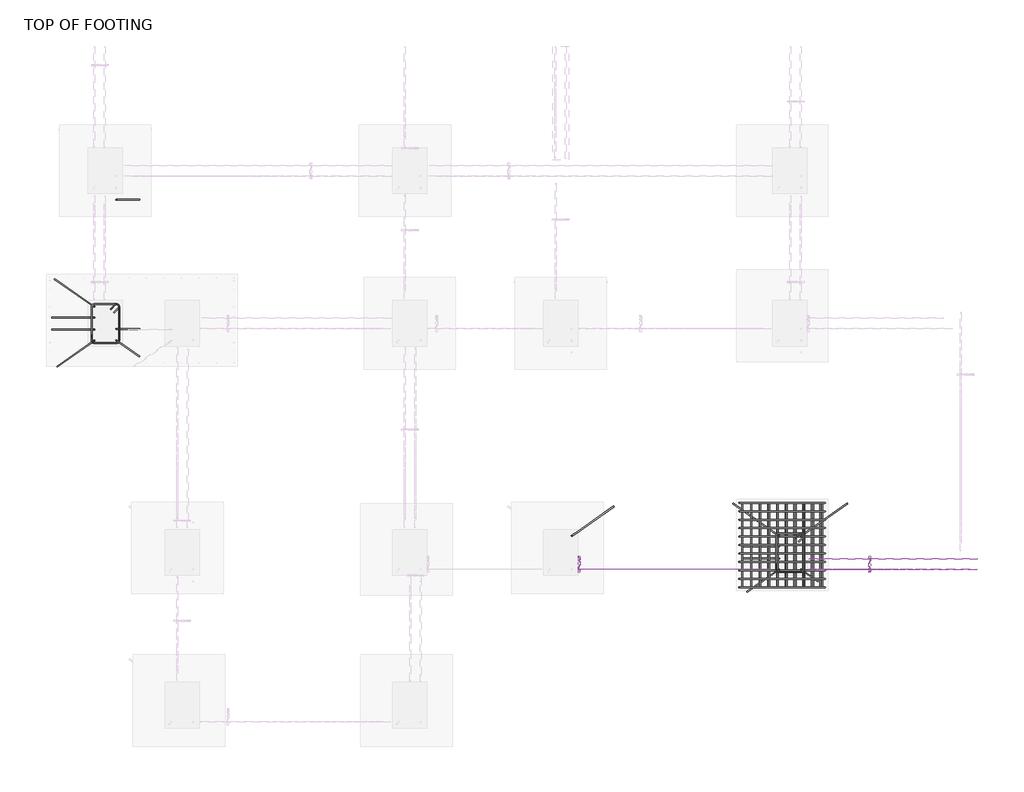
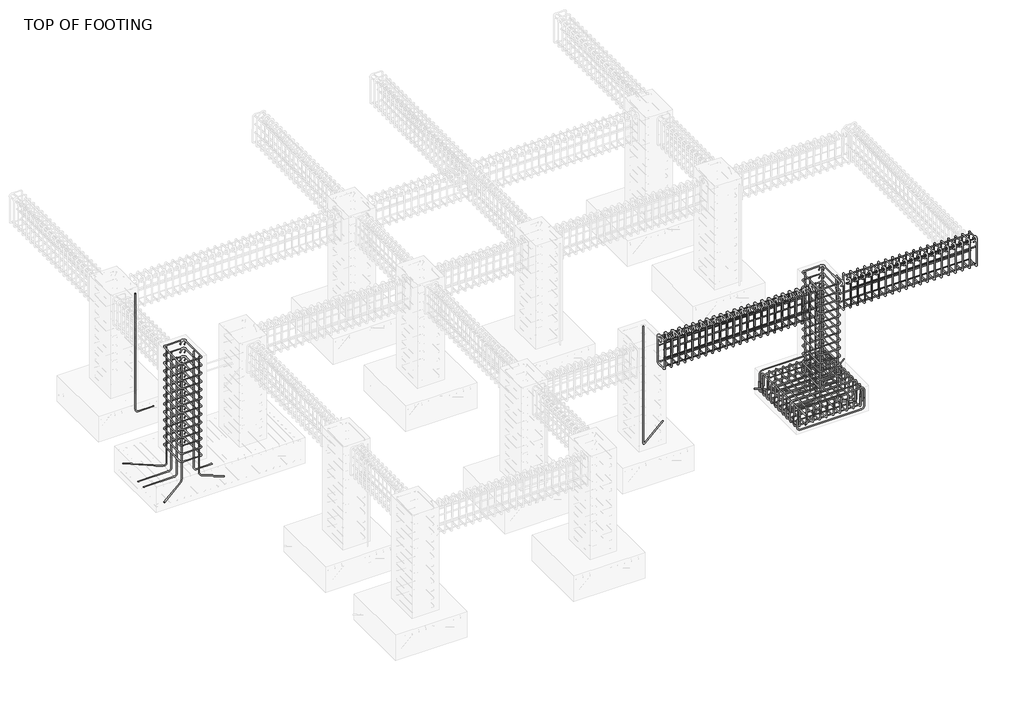
# One storey, part 5 of 17: 27 reinforcing bars.
"""IFC4 building model written with IfcOpenShell, lengths in millimetres."""

from ifc_helpers import new_model, si_unit, point, frame, origin, place, context, project, spatial, polyline, circle_curve, trimmed, segment, composite_curve, source, transform, mapped, element, save
from ifc_brep_helpers import swept_disk

model = new_model("IFC4")

# Units and contexts
model_context = context("Model", 3, world=origin())
ifc_project = project(units=[si_unit("LENGTHUNIT", "METRE", prefix="MILLI")], contexts=[model_context])

# Site, building, storey
site = spatial("IfcSite", under=ifc_project)
building = spatial("IfcBuilding", under=site)
storey = spatial("IfcBuildingStorey", under=building, Name="TOP OF FOOTING", Elevation=-1828.8)

# Reinforcing bars
placement = place(None, origin())
reinforcing_bar_shape = source(origin(), model_context, "Body", "SolidModel", [
    swept_disk(composite_curve([segment(polyline([(5115.7588658, -280.8742842, -2051.4362487), (5115.7588658, -280.8742842, -2198.7362487)]), True, "CONTINUOUS"), segment(trimmed(circle_curve(frame((5069.4088658, -280.8742842, -2198.7362487), z_axis=(0.0, 1.0, 0.0), x_axis=(46.350000000000364, 0.0, 0.0)), 46.35), [point((5115.7588658, -280.8742842, -2198.7362487))], [point((5069.4088658, -280.8742842, -2245.0862487))], True, "CARTESIAN"), True, "CONTINUOUS"), segment(polyline([(5069.4088658, -280.8742842, -2245.0862487), (4044.0910413, -280.8742842, -2245.0862487)]), True, "CONTINUOUS"), segment(trimmed(circle_curve(frame((4044.0910413, -280.8742842, -2198.7362487), z_axis=(0.0, 1.0, 0.0), x_axis=(0.0, 0.0, -46.34999999999991)), 46.35), [point((4044.0910413, -280.8742842, -2245.0862487))], [point((3997.7410413, -280.8742842, -2198.7362487))], True, "CARTESIAN"), True, "CONTINUOUS"), segment(polyline([(3997.7410413, -280.8742842, -2198.7362487), (3997.7410413, -280.8742842, -2051.4362487)]), True, "CONTINUOUS")], self_intersect=False), 6.35),
])
element("IfcReinforcingBar", 1, at=placement, inside=storey, context=model_context, shape_type="MappedRepresentation", body=[
    mapped(reinforcing_bar_shape, transform((0.0, 0.0, 0.0), x_axis=(1.0, 0.0, 0.0), y_axis=(0.0, 1.0, 0.0), z_axis=(0.0, 0.0, 1.0))),
    mapped(reinforcing_bar_shape, transform((0.0, -110.73, 0.0), x_axis=(1.0, 0.0, 0.0), y_axis=(0.0, 1.0, 0.0), z_axis=(0.0, 0.0, 1.0))),
    mapped(reinforcing_bar_shape, transform((0.0, -221.46, 0.0), x_axis=(1.0, 0.0, 0.0), y_axis=(0.0, 1.0, 0.0), z_axis=(0.0, 0.0, 1.0))),
    mapped(reinforcing_bar_shape, transform((0.0, -332.19, 0.0), x_axis=(1.0, 0.0, 0.0), y_axis=(0.0, 1.0, 0.0), z_axis=(0.0, 0.0, 1.0))),
    mapped(reinforcing_bar_shape, transform((0.0, -442.92, 0.0), x_axis=(1.0, 0.0, 0.0), y_axis=(0.0, 1.0, 0.0), z_axis=(0.0, 0.0, 1.0))),
    mapped(reinforcing_bar_shape, transform((0.0, -553.65, 0.0), x_axis=(1.0, 0.0, 0.0), y_axis=(0.0, 1.0, 0.0), z_axis=(0.0, 0.0, 1.0))),
    mapped(reinforcing_bar_shape, transform((0.0, -664.38, 0.0), x_axis=(1.0, 0.0, 0.0), y_axis=(0.0, 1.0, 0.0), z_axis=(0.0, 0.0, 1.0))),
    mapped(reinforcing_bar_shape, transform((0.0, -775.11, 0.0), x_axis=(1.0, 0.0, 0.0), y_axis=(0.0, 1.0, 0.0), z_axis=(0.0, 0.0, 1.0))),
    mapped(reinforcing_bar_shape, transform((0.0, -885.84, 0.0), x_axis=(1.0, 0.0, 0.0), y_axis=(0.0, 1.0, 0.0), z_axis=(0.0, 0.0, 1.0))),
    mapped(reinforcing_bar_shape, transform((0.0, -996.57, 0.0), x_axis=(1.0, 0.0, 0.0), y_axis=(0.0, 1.0, 0.0), z_axis=(0.0, 0.0, 1.0))),
    mapped(reinforcing_bar_shape, transform((0.0, -1107.3, 0.0), x_axis=(1.0, 0.0, 0.0), y_axis=(0.0, 1.0, 0.0), z_axis=(0.0, 0.0, 1.0))),
])
reinforcing_bar_2_shape = source(origin(), model_context, "Body", "SolidModel", [
    swept_disk(composite_curve([segment(polyline([(4008.404705, -280.8742842, -2058.517229), (4008.404705, -280.8742842, -1911.217229)]), True, "CONTINUOUS"), segment(trimmed(circle_curve(frame((4054.754705, -280.8742842, -1911.217229), z_axis=(0.0, 1.0, 0.0), x_axis=(-46.34999999999991, 0.0, 0.0)), 46.35), [point((4008.404705, -280.8742842, -1911.217229))], [point((4054.754705, -280.8742842, -1864.867229))], True, "CARTESIAN"), True, "CONTINUOUS"), segment(polyline([(4054.754705, -280.8742842, -1864.867229), (5073.3110915, -280.8742842, -1864.867229)]), True, "CONTINUOUS"), segment(trimmed(circle_curve(frame((5073.3110915, -280.8742842, -1911.217229), z_axis=(0.0, 1.0, 0.0), x_axis=(0.0, 0.0, 46.350000000000136)), 46.35), [point((5073.3110915, -280.8742842, -1864.867229))], [point((5119.6610915, -280.8742842, -1911.217229))], True, "CARTESIAN"), True, "CONTINUOUS"), segment(polyline([(5119.6610915, -280.8742842, -1911.217229), (5119.6610915, -280.8742842, -2058.517229)]), True, "CONTINUOUS")], self_intersect=False), 6.35),
])
element("IfcReinforcingBar", 2, at=placement, inside=storey, context=model_context, shape_type="MappedRepresentation", body=[
    mapped(reinforcing_bar_2_shape, transform((0.0, 0.0, 0.0), x_axis=(1.0, 0.0, 0.0), y_axis=(0.0, 1.0, 0.0), z_axis=(0.0, 0.0, 1.0))),
    mapped(reinforcing_bar_2_shape, transform((0.0, -110.73, 0.0), x_axis=(1.0, 0.0, 0.0), y_axis=(0.0, 1.0, 0.0), z_axis=(0.0, 0.0, 1.0))),
    mapped(reinforcing_bar_2_shape, transform((0.0, -221.46, 0.0), x_axis=(1.0, 0.0, 0.0), y_axis=(0.0, 1.0, 0.0), z_axis=(0.0, 0.0, 1.0))),
    mapped(reinforcing_bar_2_shape, transform((0.0, -332.19, 0.0), x_axis=(1.0, 0.0, 0.0), y_axis=(0.0, 1.0, 0.0), z_axis=(0.0, 0.0, 1.0))),
    mapped(reinforcing_bar_2_shape, transform((0.0, -442.92, 0.0), x_axis=(1.0, 0.0, 0.0), y_axis=(0.0, 1.0, 0.0), z_axis=(0.0, 0.0, 1.0))),
    mapped(reinforcing_bar_2_shape, transform((0.0, -553.65, 0.0), x_axis=(1.0, 0.0, 0.0), y_axis=(0.0, 1.0, 0.0), z_axis=(0.0, 0.0, 1.0))),
    mapped(reinforcing_bar_2_shape, transform((0.0, -664.38, 0.0), x_axis=(1.0, 0.0, 0.0), y_axis=(0.0, 1.0, 0.0), z_axis=(0.0, 0.0, 1.0))),
    mapped(reinforcing_bar_2_shape, transform((0.0, -775.11, 0.0), x_axis=(1.0, 0.0, 0.0), y_axis=(0.0, 1.0, 0.0), z_axis=(0.0, 0.0, 1.0))),
    mapped(reinforcing_bar_2_shape, transform((0.0, -885.84, 0.0), x_axis=(1.0, 0.0, 0.0), y_axis=(0.0, 1.0, 0.0), z_axis=(0.0, 0.0, 1.0))),
    mapped(reinforcing_bar_2_shape, transform((0.0, -996.57, 0.0), x_axis=(1.0, 0.0, 0.0), y_axis=(0.0, 1.0, 0.0), z_axis=(0.0, 0.0, 1.0))),
    mapped(reinforcing_bar_2_shape, transform((0.0, -1107.3, 0.0), x_axis=(1.0, 0.0, 0.0), y_axis=(0.0, 1.0, 0.0), z_axis=(0.0, 0.0, 1.0))),
])
reinforcing_bar_3_shape = source(origin(), model_context, "Body", "SolidModel", [
    swept_disk(composite_curve([segment(polyline([(5082.6693864, -280.8742842, -2093.0974099), (5082.6693864, -280.8742842, -1945.7974099)]), True, "CONTINUOUS"), segment(trimmed(circle_curve(frame((5082.6693864, -327.2242842, -1945.7974099), z_axis=(1.0, 0.0, 0.0), x_axis=(0.0, 46.35000000000002, 0.0)), 46.35), [point((5082.6693864, -280.8742842, -1945.7974099))], [point((5082.6693864, -327.2242842, -1899.4474099))], True, "CARTESIAN"), True, "CONTINUOUS"), segment(polyline([(5082.6693864, -327.2242842, -1899.4474099), (5082.6693864, -1341.8242842, -1899.4474099)]), True, "CONTINUOUS"), segment(trimmed(circle_curve(frame((5082.6693864, -1341.8242842, -1945.7974099), z_axis=(1.0, 0.0, 0.0), x_axis=(0.0, 0.0, 46.350000000000136)), 46.35), [point((5082.6693864, -1341.8242842, -1899.4474099))], [point((5082.6693864, -1388.1742842, -1945.7974099))], True, "CARTESIAN"), True, "CONTINUOUS"), segment(polyline([(5082.6693864, -1388.1742842, -1945.7974099), (5082.6693864, -1388.1742842, -2093.0974099)]), True, "CONTINUOUS")], self_intersect=False), 6.35),
])
element("IfcReinforcingBar", 3, at=placement, inside=storey, context=model_context, shape_type="MappedRepresentation", body=[
    mapped(reinforcing_bar_3_shape, transform((0.0, 0.0, 0.0), x_axis=(1.0, 0.0, 0.0), y_axis=(0.0, 1.0, 0.0), z_axis=(0.0, 0.0, 1.0))),
    mapped(reinforcing_bar_3_shape, transform((-115.9606781, 0.0, 0.0), x_axis=(1.0, 0.0, 0.0), y_axis=(0.0, 1.0, 0.0), z_axis=(0.0, 0.0, 1.0))),
    mapped(reinforcing_bar_3_shape, transform((-231.9213561, 0.0, 0.0), x_axis=(1.0, 0.0, 0.0), y_axis=(0.0, 1.0, 0.0), z_axis=(0.0, 0.0, 1.0))),
    mapped(reinforcing_bar_3_shape, transform((-347.8820342, 0.0, 0.0), x_axis=(1.0, 0.0, 0.0), y_axis=(0.0, 1.0, 0.0), z_axis=(0.0, 0.0, 1.0))),
    mapped(reinforcing_bar_3_shape, transform((-463.8427123, 0.0, 0.0), x_axis=(1.0, 0.0, 0.0), y_axis=(0.0, 1.0, 0.0), z_axis=(0.0, 0.0, 1.0))),
    mapped(reinforcing_bar_3_shape, transform((-579.8033904, 0.0, 0.0), x_axis=(1.0, 0.0, 0.0), y_axis=(0.0, 1.0, 0.0), z_axis=(0.0, 0.0, 1.0))),
    mapped(reinforcing_bar_3_shape, transform((-695.7640684, 0.0, 0.0), x_axis=(1.0, 0.0, 0.0), y_axis=(0.0, 1.0, 0.0), z_axis=(0.0, 0.0, 1.0))),
    mapped(reinforcing_bar_3_shape, transform((-811.7247465, 0.0, 0.0), x_axis=(1.0, 0.0, 0.0), y_axis=(0.0, 1.0, 0.0), z_axis=(0.0, 0.0, 1.0))),
    mapped(reinforcing_bar_3_shape, transform((-927.6854246, 0.0, 0.0), x_axis=(1.0, 0.0, 0.0), y_axis=(0.0, 1.0, 0.0), z_axis=(0.0, 0.0, 1.0))),
    mapped(reinforcing_bar_3_shape, transform((-1043.6461027, 0.0, 0.0), x_axis=(1.0, 0.0, 0.0), y_axis=(0.0, 1.0, 0.0), z_axis=(0.0, 0.0, 1.0))),
])
reinforcing_bar_4_shape = source(origin(), model_context, "Body", "SolidModel", [
    swept_disk(composite_curve([segment(polyline([(4039.0232837, -280.8742842, -2009.4698822), (4039.0232837, -280.8742842, -2156.7698822)]), True, "CONTINUOUS"), segment(trimmed(circle_curve(frame((4039.0232837, -327.2242842, -2156.7698822), z_axis=(-1.0, 0.0, 0.0), x_axis=(0.0, 46.35000000000002, 0.0)), 46.35), [point((4039.0232837, -280.8742842, -2156.7698822))], [point((4039.0232837, -327.2242842, -2203.1198822))], True, "CARTESIAN"), True, "CONTINUOUS"), segment(polyline([(4039.0232837, -327.2242842, -2203.1198822), (4039.0232837, -1341.8242842, -2203.1198822)]), True, "CONTINUOUS"), segment(trimmed(circle_curve(frame((4039.0232837, -1341.8242842, -2156.7698822), z_axis=(-1.0, 0.0, 0.0), x_axis=(0.0, 0.0, -46.34999999999991)), 46.35), [point((4039.0232837, -1341.8242842, -2203.1198822))], [point((4039.0232837, -1388.1742842, -2156.7698822))], True, "CARTESIAN"), True, "CONTINUOUS"), segment(polyline([(4039.0232837, -1388.1742842, -2156.7698822), (4039.0232837, -1388.1742842, -2009.4698822)]), True, "CONTINUOUS")], self_intersect=False), 6.35),
])
element("IfcReinforcingBar", 4, at=placement, inside=storey, context=model_context, shape_type="MappedRepresentation", body=[
    mapped(reinforcing_bar_4_shape, transform((0.0, 0.0, 0.0), x_axis=(1.0, 0.0, 0.0), y_axis=(0.0, 1.0, 0.0), z_axis=(0.0, 0.0, 1.0))),
    mapped(reinforcing_bar_4_shape, transform((113.1523491, 0.0, 0.0), x_axis=(1.0, 0.0, 0.0), y_axis=(0.0, 1.0, 0.0), z_axis=(0.0, 0.0, 1.0))),
    mapped(reinforcing_bar_4_shape, transform((226.3046983, 0.0, 0.0), x_axis=(1.0, 0.0, 0.0), y_axis=(0.0, 1.0, 0.0), z_axis=(0.0, 0.0, 1.0))),
    mapped(reinforcing_bar_4_shape, transform((339.4570474, 0.0, 0.0), x_axis=(1.0, 0.0, 0.0), y_axis=(0.0, 1.0, 0.0), z_axis=(0.0, 0.0, 1.0))),
    mapped(reinforcing_bar_4_shape, transform((452.6093966, 0.0, 0.0), x_axis=(1.0, 0.0, 0.0), y_axis=(0.0, 1.0, 0.0), z_axis=(0.0, 0.0, 1.0))),
    mapped(reinforcing_bar_4_shape, transform((565.7617457, 0.0, 0.0), x_axis=(1.0, 0.0, 0.0), y_axis=(0.0, 1.0, 0.0), z_axis=(0.0, 0.0, 1.0))),
    mapped(reinforcing_bar_4_shape, transform((678.9140949, 0.0, 0.0), x_axis=(1.0, 0.0, 0.0), y_axis=(0.0, 1.0, 0.0), z_axis=(0.0, 0.0, 1.0))),
    mapped(reinforcing_bar_4_shape, transform((792.066444, 0.0, 0.0), x_axis=(1.0, 0.0, 0.0), y_axis=(0.0, 1.0, 0.0), z_axis=(0.0, 0.0, 1.0))),
    mapped(reinforcing_bar_4_shape, transform((905.2187932, 0.0, 0.0), x_axis=(1.0, 0.0, 0.0), y_axis=(0.0, 1.0, 0.0), z_axis=(0.0, 0.0, 1.0))),
    mapped(reinforcing_bar_4_shape, transform((1018.3711423, 0.0, 0.0), x_axis=(1.0, 0.0, 0.0), y_axis=(0.0, 1.0, 0.0), z_axis=(0.0, 0.0, 1.0))),
])
reinforcing_bar_5_shape = source(origin(), model_context, "Body", "SolidModel", [
    swept_disk(composite_curve([segment(polyline([(-4230.403382, 2254.1999505, -46.35), (-4174.6598191, 2309.9435134, -46.35)]), True, "CONTINUOUS"), segment(trimmed(circle_curve(frame((-4152.4920215, 2287.7757158, -46.35), z_axis=(0.0, 0.0, -1.0), x_axis=(-22.167797600000085, 22.167797600000085, 0.0)), 31.35), [point((-4174.6598191, 2309.9435134, -46.35))], [point((-4121.1420215, 2287.7757158, -46.35))], True, "CARTESIAN"), True, "CONTINUOUS"), segment(polyline([(-4121.1420215, 2287.7757158, -46.35), (-4121.1420215, 1843.1757158, -46.35)]), True, "CONTINUOUS"), segment(trimmed(circle_curve(frame((-4152.4920215, 1843.1757158, -46.35), z_axis=(0.0, 0.0, -1.0), x_axis=(31.350000000000364, 0.0, 0.0)), 31.35), [point((-4121.1420215, 1843.1757158, -46.35))], [point((-4152.4920215, 1811.8257158, -46.35))], True, "CARTESIAN"), True, "CONTINUOUS"), segment(polyline([(-4152.4920215, 1811.8257158, -46.35), (-4447.0920215, 1811.8257158, -46.35)]), True, "CONTINUOUS"), segment(trimmed(circle_curve(frame((-4447.0920215, 1843.1658965, -45.5654144), z_axis=(0.0, 0.025026655153786343, -0.9996867842138424), x_axis=(0.0, -31.34018070000002, -0.7845855999999998)), 31.35), [point((-4447.0920215, 1811.8257158, -46.35))], [point((-4478.4420215, 1843.1658965, -45.5654144))], True, "CARTESIAN"), True, "CONTINUOUS"), segment(polyline([(-4478.4420215, 1843.1658965, -45.5654144), (-4478.4420215, 2287.7855351, -34.4345856)]), True, "CONTINUOUS"), segment(trimmed(circle_curve(frame((-4447.0920215, 2287.7855351, -34.4345856), z_axis=(0.0, 0.025026655153786343, -0.9996867842138424), x_axis=(-31.350000000000364, 0.0, 0.0)), 31.35), [point((-4478.4420215, 2287.7855351, -34.4345856))], [point((-4447.0920215, 2319.1257158, -33.65))], True, "CARTESIAN"), True, "CONTINUOUS"), segment(polyline([(-4447.0920215, 2319.1257158, -33.65), (-4152.4920215, 2319.1257158, -33.65)]), True, "CONTINUOUS"), segment(trimmed(circle_curve(frame((-4152.4920215, 2287.7757158, -33.65), z_axis=(0.0, 0.0, -1.0), x_axis=(0.0, 31.34999999999991, 0.0)), 31.35), [point((-4152.4920215, 2319.1257158, -33.65))], [point((-4130.3242239, 2265.6079182, -33.65))], True, "CARTESIAN"), True, "CONTINUOUS"), segment(polyline([(-4130.3242239, 2265.6079182, -33.65), (-4186.0677868, 2209.8643553, -33.65)]), True, "CONTINUOUS")], self_intersect=False), 6.35),
])
element("IfcReinforcingBar", 5, at=placement, inside=storey, context=model_context, shape_type="MappedRepresentation", body=[
    mapped(reinforcing_bar_5_shape, transform((0.0, 0.0, 0.0), x_axis=(1.0, 0.0, 0.0), y_axis=(0.0, 1.0, 0.0), z_axis=(0.0, 0.0, 1.0))),
    mapped(reinforcing_bar_5_shape, transform((0.0, 0.0, -144.675), x_axis=(1.0, 0.0, 0.0), y_axis=(0.0, 1.0, 0.0), z_axis=(0.0, 0.0, 1.0))),
    mapped(reinforcing_bar_5_shape, transform((0.0, 0.0, -289.35), x_axis=(1.0, 0.0, 0.0), y_axis=(0.0, 1.0, 0.0), z_axis=(0.0, 0.0, 1.0))),
    mapped(reinforcing_bar_5_shape, transform((0.0, 0.0, -434.025), x_axis=(1.0, 0.0, 0.0), y_axis=(0.0, 1.0, 0.0), z_axis=(0.0, 0.0, 1.0))),
    mapped(reinforcing_bar_5_shape, transform((0.0, 0.0, -578.7), x_axis=(1.0, 0.0, 0.0), y_axis=(0.0, 1.0, 0.0), z_axis=(0.0, 0.0, 1.0))),
    mapped(reinforcing_bar_5_shape, transform((0.0, 0.0, -723.375), x_axis=(1.0, 0.0, 0.0), y_axis=(0.0, 1.0, 0.0), z_axis=(0.0, 0.0, 1.0))),
    mapped(reinforcing_bar_5_shape, transform((0.0, 0.0, -868.05), x_axis=(1.0, 0.0, 0.0), y_axis=(0.0, 1.0, 0.0), z_axis=(0.0, 0.0, 1.0))),
    mapped(reinforcing_bar_5_shape, transform((0.0, 0.0, -1012.725), x_axis=(1.0, 0.0, 0.0), y_axis=(0.0, 1.0, 0.0), z_axis=(0.0, 0.0, 1.0))),
    mapped(reinforcing_bar_5_shape, transform((0.0, 0.0, -1157.4), x_axis=(1.0, 0.0, 0.0), y_axis=(0.0, 1.0, 0.0), z_axis=(0.0, 0.0, 1.0))),
    mapped(reinforcing_bar_5_shape, transform((0.0, 0.0, -1302.075), x_axis=(1.0, 0.0, 0.0), y_axis=(0.0, 1.0, 0.0), z_axis=(0.0, 0.0, 1.0))),
    mapped(reinforcing_bar_5_shape, transform((0.0, 0.0, -1446.75), x_axis=(1.0, 0.0, 0.0), y_axis=(0.0, 1.0, 0.0), z_axis=(0.0, 0.0, 1.0))),
    mapped(reinforcing_bar_5_shape, transform((0.0, 0.0, -1591.425), x_axis=(1.0, 0.0, 0.0), y_axis=(0.0, 1.0, 0.0), z_axis=(0.0, 0.0, 1.0))),
    mapped(reinforcing_bar_5_shape, transform((0.0, 0.0, -1736.1), x_axis=(1.0, 0.0, 0.0), y_axis=(0.0, 1.0, 0.0), z_axis=(0.0, 0.0, 1.0))),
])
reinforcing_bar_6_shape = source(origin(), model_context, "Body", "SolidModel", [
    swept_disk(composite_curve([segment(polyline([(-4155.5276111, 1997.3689995, -40.0), (-4155.5276111, 1997.3689995, -2094.5391135)]), True, "CONTINUOUS"), segment(trimmed(circle_curve(frame((-4109.1776111, 1997.3689995, -2094.5391135), z_axis=(0.0, -1.0, 0.0), x_axis=(-46.350000000000364, 0.0, 0.0)), 46.35), [point((-4155.5276111, 1997.3689995, -2094.5391135))], [point((-4109.1776111, 1997.3689995, -2140.8891135))], True, "CARTESIAN"), True, "CONTINUOUS"), segment(polyline([(-4109.1776111, 1997.3689995, -2140.8891135), (-3849.2038294, 1997.3689995, -2140.8891135)]), True, "CONTINUOUS")], self_intersect=False), 6.35),
])
element("IfcReinforcingBar", 6, at=placement, inside=storey, context=model_context, shape_type="MappedRepresentation", body=[
    mapped(reinforcing_bar_6_shape, transform((0.0, 0.0, 0.0), x_axis=(1.0, 0.0, 0.0), y_axis=(0.0, 1.0, 0.0), z_axis=(0.0, 0.0, 1.0))),
    mapped(reinforcing_bar_6_shape, transform((0.0, 1690.7260472, 0.0), x_axis=(1.0, 0.0, 0.0), y_axis=(0.0, 1.0, 0.0), z_axis=(0.0, 0.0, 1.0))),
])
element("IfcReinforcingBar", 7, at=placement, inside=storey, context=model_context, shape_type="SolidModel", body=[
    swept_disk(composite_curve([segment(polyline([(-4444.0564318, 2286.4257158, -40.0), (-4444.0564318, 2286.4257158, -2094.5391135)]), True, "CONTINUOUS"), segment(trimmed(circle_curve(frame((-4482.0241291, 2313.0109836, -2094.5391135), z_axis=(0.5735764363510419, 0.8191520442889948, 0.0), x_axis=(37.96769730000051, -26.58526780000011, 0.0)), 46.35), [point((-4444.0564318, 2286.4257158, -2094.5391135))], [point((-4482.0241291, 2313.0109836, -2140.8891135))], True, "CARTESIAN"), True, "CONTINUOUS"), segment(polyline([(-4482.0241291, 2313.0109836, -2140.8891135), (-4963.5335446, 2650.1675061, -2140.8891135)]), True, "CONTINUOUS")], self_intersect=False), 6.35),
])
element("IfcReinforcingBar", 8, at=placement, inside=storey, context=model_context, shape_type="SolidModel", body=[
    swept_disk(composite_curve([segment(polyline([(-4155.5276111, 1844.5257158, -40.0), (-4155.5276111, 1844.5257158, -2094.5391135)]), True, "CONTINUOUS"), segment(trimmed(circle_curve(frame((-4117.5599139, 1817.940448, -2094.5391135), z_axis=(-0.5735764363510363, -0.8191520442889988, 0.0), x_axis=(-37.96769720000066, 26.585267799999883, 0.0)), 46.35), [point((-4155.5276111, 1844.5257158, -2094.5391135))], [point((-4117.5599139, 1817.940448, -2140.8891135))], True, "CARTESIAN"), True, "CONTINUOUS"), segment(polyline([(-4117.5599139, 1817.940448, -2140.8891135), (-3853.7755504, 1633.2366482, -2140.8891135)]), True, "CONTINUOUS")], self_intersect=False), 6.35),
])
element("IfcReinforcingBar", 9, at=placement, inside=storey, context=model_context, shape_type="SolidModel", body=[
    swept_disk(composite_curve([segment(polyline([(-4444.0564318, 1844.5257158, -40.0), (-4444.0564318, 1844.5257158, -2094.5391135)]), True, "CONTINUOUS"), segment(trimmed(circle_curve(frame((-4482.0241291, 1817.940448, -2094.5391135), z_axis=(-0.5735764363510419, 0.8191520442889948, 0.0), x_axis=(37.96769730000051, 26.585267799999883, 0.0)), 46.35), [point((-4444.0564318, 1844.5257158, -2094.5391135))], [point((-4482.0241291, 1817.940448, -2140.8891135))], True, "CARTESIAN"), True, "CONTINUOUS"), segment(polyline([(-4482.0241291, 1817.940448, -2140.8891135), (-4933.5928236, 1501.748644, -2140.8891135)]), True, "CONTINUOUS")], self_intersect=False), 6.35),
])
reinforcing_bar_7_shape = source(origin(), model_context, "Body", "SolidModel", [
    swept_disk(composite_curve([segment(polyline([(-4444.0564318, 2147.3689995, -40.0), (-4444.0564318, 2147.3689995, -2094.5391135)]), True, "CONTINUOUS"), segment(trimmed(circle_curve(frame((-4490.4064318, 2147.3689995, -2094.5391135), z_axis=(0.0, 1.0, 0.0), x_axis=(46.350000000000364, 0.0, 0.0)), 46.35), [point((-4444.0564318, 2147.3689995, -2094.5391135))], [point((-4490.4064318, 2147.3689995, -2140.8891135))], True, "CARTESIAN"), True, "CONTINUOUS"), segment(polyline([(-4490.4064318, 2147.3689995, -2140.8891135), (-5004.1383392, 2147.3689995, -2140.8891135)]), True, "CONTINUOUS")], self_intersect=False), 6.35),
])
element("IfcReinforcingBar", 10, at=placement, inside=storey, context=model_context, shape_type="MappedRepresentation", body=[
    mapped(reinforcing_bar_7_shape, transform((0.0, 0.0, 0.0), x_axis=(1.0, 0.0, 0.0), y_axis=(0.0, 1.0, 0.0), z_axis=(0.0, 0.0, 1.0))),
    mapped(reinforcing_bar_7_shape, transform((0.0, -159.2739528, 0.0), x_axis=(1.0, 0.0, 0.0), y_axis=(0.0, 1.0, 0.0), z_axis=(0.0, 0.0, 1.0))),
])
element("IfcReinforcingBar", 11, at=placement, inside=storey, context=model_context, shape_type="SolidModel", body=[
    swept_disk(composite_curve([segment(polyline([(1806.3732761, -713.5742842, -40.0), (1806.3732761, -713.5742842, -2094.5391135)]), True, "CONTINUOUS"), segment(trimmed(circle_curve(frame((1844.3409734, -686.9890164, -2094.5391135), z_axis=(0.5735764363510363, -0.8191520442889988, 0.0), x_axis=(-37.96769729999983, -26.585267799999997, 0.0)), 46.35), [point((1806.3732761, -713.5742842, -2094.5391135))], [point((1844.3409734, -686.9890164, -2140.8891135))], True, "CARTESIAN"), True, "CONTINUOUS"), segment(polyline([(1844.3409734, -686.9890164, -2140.8891135), (2354.4133491, -329.8324939, -2140.8891135)]), True, "CONTINUOUS")], self_intersect=False), 6.35),
])
reinforcing_bar_8_shape = source(origin(), model_context, "Body", "SolidModel", [
    swept_disk(composite_curve([segment(polyline([(4731.4975053, -745.8000495, -46.35), (4787.2410682, -690.0564866, -46.35)]), True, "CONTINUOUS"), segment(trimmed(circle_curve(frame((4809.4088658, -712.2242842, -46.35), z_axis=(0.0, 0.0, -1.0), x_axis=(-22.167797600000085, 22.167797600000085, 0.0)), 31.35), [point((4787.2410682, -690.0564866, -46.35))], [point((4840.7588658, -712.2242842, -46.35))], True, "CARTESIAN"), True, "CONTINUOUS"), segment(polyline([(4840.7588658, -712.2242842, -46.35), (4840.7588658, -1156.8242842, -46.35)]), True, "CONTINUOUS"), segment(trimmed(circle_curve(frame((4809.4088658, -1156.8242842, -46.35), z_axis=(0.0, 0.0, -1.0), x_axis=(31.350000000000364, 0.0, 0.0)), 31.35), [point((4840.7588658, -1156.8242842, -46.35))], [point((4809.4088658, -1188.1742842, -46.35))], True, "CARTESIAN"), True, "CONTINUOUS"), segment(polyline([(4809.4088658, -1188.1742842, -46.35), (4514.8088658, -1188.1742842, -46.35)]), True, "CONTINUOUS"), segment(trimmed(circle_curve(frame((4514.8088658, -1156.8341035, -45.5654144), z_axis=(0.0, 0.025026655153786343, -0.9996867842138424), x_axis=(0.0, -31.34018070000002, -0.7845855999999998)), 31.35), [point((4514.8088658, -1188.1742842, -46.35))], [point((4483.4588658, -1156.8341035, -45.5654144))], True, "CARTESIAN"), True, "CONTINUOUS"), segment(polyline([(4483.4588658, -1156.8341035, -45.5654144), (4483.4588658, -712.2144649, -34.4345856)]), True, "CONTINUOUS"), segment(trimmed(circle_curve(frame((4514.8088658, -712.2144649, -34.4345856), z_axis=(0.0, 0.025026655153786343, -0.9996867842138424), x_axis=(-31.349999999999454, 0.0, 0.0)), 31.35), [point((4483.4588658, -712.2144649, -34.4345856))], [point((4514.8088658, -680.8742842, -33.65))], True, "CARTESIAN"), True, "CONTINUOUS"), segment(polyline([(4514.8088658, -680.8742842, -33.65), (4809.4088658, -680.8742842, -33.65)]), True, "CONTINUOUS"), segment(trimmed(circle_curve(frame((4809.4088658, -712.2242842, -33.65), z_axis=(0.0, 0.0, -1.0), x_axis=(0.0, 31.350000000000023, 0.0)), 31.35), [point((4809.4088658, -680.8742842, -33.65))], [point((4831.5766634, -734.3920818, -33.65))], True, "CARTESIAN"), True, "CONTINUOUS"), segment(polyline([(4831.5766634, -734.3920818, -33.65), (4775.8331004, -790.1356447, -33.65)]), True, "CONTINUOUS")], self_intersect=False), 6.35),
])
element("IfcReinforcingBar", 12, at=placement, inside=storey, context=model_context, shape_type="MappedRepresentation", body=[
    mapped(reinforcing_bar_8_shape, transform((0.0, 0.0, 0.0), x_axis=(1.0, 0.0, 0.0), y_axis=(0.0, 1.0, 0.0), z_axis=(0.0, 0.0, 1.0))),
    mapped(reinforcing_bar_8_shape, transform((0.0, 0.0, -144.675), x_axis=(1.0, 0.0, 0.0), y_axis=(0.0, 1.0, 0.0), z_axis=(0.0, 0.0, 1.0))),
    mapped(reinforcing_bar_8_shape, transform((0.0, 0.0, -289.35), x_axis=(1.0, 0.0, 0.0), y_axis=(0.0, 1.0, 0.0), z_axis=(0.0, 0.0, 1.0))),
    mapped(reinforcing_bar_8_shape, transform((0.0, 0.0, -434.025), x_axis=(1.0, 0.0, 0.0), y_axis=(0.0, 1.0, 0.0), z_axis=(0.0, 0.0, 1.0))),
    mapped(reinforcing_bar_8_shape, transform((0.0, 0.0, -578.7), x_axis=(1.0, 0.0, 0.0), y_axis=(0.0, 1.0, 0.0), z_axis=(0.0, 0.0, 1.0))),
    mapped(reinforcing_bar_8_shape, transform((0.0, 0.0, -723.375), x_axis=(1.0, 0.0, 0.0), y_axis=(0.0, 1.0, 0.0), z_axis=(0.0, 0.0, 1.0))),
    mapped(reinforcing_bar_8_shape, transform((0.0, 0.0, -868.05), x_axis=(1.0, 0.0, 0.0), y_axis=(0.0, 1.0, 0.0), z_axis=(0.0, 0.0, 1.0))),
    mapped(reinforcing_bar_8_shape, transform((0.0, 0.0, -1012.725), x_axis=(1.0, 0.0, 0.0), y_axis=(0.0, 1.0, 0.0), z_axis=(0.0, 0.0, 1.0))),
    mapped(reinforcing_bar_8_shape, transform((0.0, 0.0, -1157.4), x_axis=(1.0, 0.0, 0.0), y_axis=(0.0, 1.0, 0.0), z_axis=(0.0, 0.0, 1.0))),
    mapped(reinforcing_bar_8_shape, transform((0.0, 0.0, -1302.075), x_axis=(1.0, 0.0, 0.0), y_axis=(0.0, 1.0, 0.0), z_axis=(0.0, 0.0, 1.0))),
    mapped(reinforcing_bar_8_shape, transform((0.0, 0.0, -1446.75), x_axis=(1.0, 0.0, 0.0), y_axis=(0.0, 1.0, 0.0), z_axis=(0.0, 0.0, 1.0))),
    mapped(reinforcing_bar_8_shape, transform((0.0, 0.0, -1591.425), x_axis=(1.0, 0.0, 0.0), y_axis=(0.0, 1.0, 0.0), z_axis=(0.0, 0.0, 1.0))),
    mapped(reinforcing_bar_8_shape, transform((0.0, 0.0, -1736.1), x_axis=(1.0, 0.0, 0.0), y_axis=(0.0, 1.0, 0.0), z_axis=(0.0, 0.0, 1.0))),
])
element("IfcReinforcingBar", 13, at=placement, inside=storey, context=model_context, shape_type="SolidModel", body=[
    swept_disk(composite_curve([segment(polyline([(4806.3732761, -713.5742842, -40.0), (4806.3732761, -713.5742842, -2094.5391135)]), True, "CONTINUOUS"), segment(trimmed(circle_curve(frame((4844.3409734, -686.9890164, -2094.5391135), z_axis=(0.5735764363510363, -0.8191520442889988, 0.0), x_axis=(-37.9676972999996, -26.585267799999997, 0.0)), 46.35), [point((4806.3732761, -713.5742842, -2094.5391135))], [point((4844.3409734, -686.9890164, -2140.8891135))], True, "CARTESIAN"), True, "CONTINUOUS"), segment(polyline([(4844.3409734, -686.9890164, -2140.8891135), (5411.5392693, -289.8324939, -2140.8891135)]), True, "CONTINUOUS")], self_intersect=False), 6.35),
])
element("IfcReinforcingBar", 14, at=placement, inside=storey, context=model_context, shape_type="SolidModel", body=[
    swept_disk(composite_curve([segment(polyline([(4517.8444555, -713.5742842, -40.0), (4517.8444555, -713.5742842, -2094.5391135)]), True, "CONTINUOUS"), segment(trimmed(circle_curve(frame((4479.8767582, -686.9890164, -2094.5391135), z_axis=(0.5735764363510419, 0.8191520442889948, 0.0), x_axis=(37.9676972999996, -26.585267799999997, 0.0)), 46.35), [point((4517.8444555, -713.5742842, -2094.5391135))], [point((4479.8767582, -686.9890164, -2140.8891135))], True, "CARTESIAN"), True, "CONTINUOUS"), segment(polyline([(4479.8767582, -686.9890164, -2140.8891135), (3912.6784623, -289.8324939, -2140.8891135)]), True, "CONTINUOUS")], self_intersect=False), 6.35),
])
element("IfcReinforcingBar", 15, at=placement, inside=storey, context=model_context, shape_type="SolidModel", body=[
    swept_disk(composite_curve([segment(polyline([(4806.3732761, -1155.4742842, -40.0), (4806.3732761, -1155.4742842, -2094.5391135)]), True, "CONTINUOUS"), segment(trimmed(circle_curve(frame((4844.3409734, -1182.059552, -2094.5391135), z_axis=(-0.5735764363510363, -0.8191520442889988, 0.0), x_axis=(-37.9676972999996, 26.585267799999883, 0.0)), 46.35), [point((4806.3732761, -1155.4742842, -2094.5391135))], [point((4844.3409734, -1182.059552, -2140.8891135))], True, "CARTESIAN"), True, "CONTINUOUS"), segment(polyline([(4844.3409734, -1182.059552, -2140.8891135), (5025.909668, -1309.1953207, -2140.8891135)]), True, "CONTINUOUS")], self_intersect=False), 6.35),
])
element("IfcReinforcingBar", 16, at=placement, inside=storey, context=model_context, shape_type="SolidModel", body=[
    swept_disk(composite_curve([segment(polyline([(4517.8444555, -1155.4742842, -40.0), (4517.8444555, -1155.4742842, -2094.5391135)]), True, "CONTINUOUS"), segment(trimmed(circle_curve(frame((4479.8767582, -1182.059552, -2094.5391135), z_axis=(-0.5735764363510419, 0.8191520442889948, 0.0), x_axis=(37.9676972999996, 26.585267799999883, 0.0)), 46.35), [point((4517.8444555, -1155.4742842, -2094.5391135))], [point((4479.8767582, -1182.059552, -2140.8891135))], True, "CARTESIAN"), True, "CONTINUOUS"), segment(polyline([(4479.8767582, -1182.059552, -2140.8891135), (4098.3080636, -1449.2368283, -2140.8891135)]), True, "CONTINUOUS")], self_intersect=False), 6.35),
])
reinforcing_bar_9_shape = source(origin(), model_context, "Body", "SolidModel", [
    swept_disk(composite_curve([segment(polyline([(4517.8444555, -852.6310005, -40.0), (4517.8444555, -852.6310005, -2094.5391135)]), True, "CONTINUOUS"), segment(trimmed(circle_curve(frame((4471.4944555, -852.6310005, -2094.5391135), z_axis=(0.0, 1.0, 0.0), x_axis=(46.349999999999454, 0.0, 0.0)), 46.35), [point((4517.8444555, -852.6310005, -2094.5391135))], [point((4471.4944555, -852.6310005, -2140.8891135))], True, "CARTESIAN"), True, "CONTINUOUS"), segment(polyline([(4471.4944555, -852.6310005, -2140.8891135), (4027.7625481, -852.6310005, -2140.8891135)]), True, "CONTINUOUS")], self_intersect=False), 6.35),
])
element("IfcReinforcingBar", 17, at=placement, inside=storey, context=model_context, shape_type="MappedRepresentation", body=[
    mapped(reinforcing_bar_9_shape, transform((0.0, 0.0, 0.0), x_axis=(1.0, 0.0, 0.0), y_axis=(0.0, 1.0, 0.0), z_axis=(0.0, 0.0, 1.0))),
    mapped(reinforcing_bar_9_shape, transform((0.0, -159.2739528, 0.0), x_axis=(1.0, 0.0, 0.0), y_axis=(0.0, 1.0, 0.0), z_axis=(0.0, 0.0, 1.0))),
])
reinforcing_bar_10_shape = source(origin(), model_context, "Body", "SolidModel", [
    swept_disk(composite_curve([segment(polyline([(4893.4588658, -1078.9129237, -111.2757654), (4893.4588658, -1134.6564866, -55.5322024)]), True, "CONTINUOUS"), segment(trimmed(circle_curve(frame((4893.4588658, -1156.8242842, -77.7), z_axis=(1.0, 0.0, 0.0), x_axis=(0.0, 22.167797599999858, 22.1677976)), 31.35), [point((4893.4588658, -1134.6564866, -55.5322024))], [point((4893.4588658, -1188.1742842, -77.7))], True, "CARTESIAN"), True, "CONTINUOUS"), segment(polyline([(4893.4588658, -1188.1742842, -77.7), (4893.4588658, -1188.1742842, -522.3)]), True, "CONTINUOUS"), segment(trimmed(circle_curve(frame((4893.4588658, -1156.8242842, -522.3), z_axis=(1.0, 0.0, 0.0), x_axis=(0.0, -31.350000000000136, 0.0)), 31.35), [point((4893.4588658, -1188.1742842, -522.3))], [point((4893.4588658, -1156.8242842, -553.65))], True, "CARTESIAN"), True, "CONTINUOUS"), segment(polyline([(4893.4588658, -1156.8242842, -553.65), (4893.4588658, -1012.2242842, -553.65)]), True, "CONTINUOUS"), segment(trimmed(circle_curve(frame((4892.6742802, -1012.2242842, -522.3098193), z_axis=(0.9996867842138424, 0.0, 0.025026655153786322), x_axis=(0.784585600000355, 0.0, -31.34018070000002)), 31.35), [point((4893.4588658, -1012.2242842, -553.65))], [point((4892.6742802, -980.8742842, -522.3098193))], True, "CARTESIAN"), True, "CONTINUOUS"), segment(polyline([(4892.6742802, -980.8742842, -522.3098193), (4881.5434514, -980.8742842, -77.6901807)]), True, "CONTINUOUS"), segment(trimmed(circle_curve(frame((4881.5434514, -1012.2242842, -77.6901807), z_axis=(0.9996867842138424, 0.0, 0.025026655153786322), x_axis=(0.0, 31.350000000000023, 0.0)), 31.35), [point((4881.5434514, -980.8742842, -77.6901807))], [point((4880.7588658, -1012.2242842, -46.35))], True, "CARTESIAN"), True, "CONTINUOUS"), segment(polyline([(4880.7588658, -1012.2242842, -46.35), (4880.7588658, -1156.8242842, -46.35)]), True, "CONTINUOUS"), segment(trimmed(circle_curve(frame((4880.7588658, -1156.8242842, -77.7), z_axis=(1.0, 0.0, 0.0), x_axis=(0.0, 0.0, 31.35)), 31.35), [point((4880.7588658, -1156.8242842, -46.35))], [point((4880.7588658, -1178.9920818, -99.8677976))], True, "CARTESIAN"), True, "CONTINUOUS"), segment(polyline([(4880.7588658, -1178.9920818, -99.8677976), (4880.7588658, -1123.2485188, -155.6113605)]), True, "CONTINUOUS")], self_intersect=False), 6.35),
])
element("IfcReinforcingBar", 18, at=placement, inside=storey, context=model_context, shape_type="MappedRepresentation", body=[
    mapped(reinforcing_bar_10_shape, transform((0.0, 0.0, 0.0), x_axis=(1.0, 0.0, 0.0), y_axis=(0.0, 1.0, 0.0), z_axis=(0.0, 0.0, 1.0))),
    mapped(reinforcing_bar_10_shape, transform((117.1052632, 0.0, 0.0), x_axis=(1.0, 0.0, 0.0), y_axis=(0.0, 1.0, 0.0), z_axis=(0.0, 0.0, 1.0))),
    mapped(reinforcing_bar_10_shape, transform((234.2105264, 0.0, 0.0), x_axis=(1.0, 0.0, 0.0), y_axis=(0.0, 1.0, 0.0), z_axis=(0.0, 0.0, 1.0))),
    mapped(reinforcing_bar_10_shape, transform((351.3157896, 0.0, 0.0), x_axis=(1.0, 0.0, 0.0), y_axis=(0.0, 1.0, 0.0), z_axis=(0.0, 0.0, 1.0))),
    mapped(reinforcing_bar_10_shape, transform((468.4210528, 0.0, 0.0), x_axis=(1.0, 0.0, 0.0), y_axis=(0.0, 1.0, 0.0), z_axis=(0.0, 0.0, 1.0))),
    mapped(reinforcing_bar_10_shape, transform((585.5263159, 0.0, 0.0), x_axis=(1.0, 0.0, 0.0), y_axis=(0.0, 1.0, 0.0), z_axis=(0.0, 0.0, 1.0))),
    mapped(reinforcing_bar_10_shape, transform((702.6315791, 0.0, 0.0), x_axis=(1.0, 0.0, 0.0), y_axis=(0.0, 1.0, 0.0), z_axis=(0.0, 0.0, 1.0))),
    mapped(reinforcing_bar_10_shape, transform((819.7368423, 0.0, 0.0), x_axis=(1.0, 0.0, 0.0), y_axis=(0.0, 1.0, 0.0), z_axis=(0.0, 0.0, 1.0))),
    mapped(reinforcing_bar_10_shape, transform((936.8421055, 0.0, 0.0), x_axis=(1.0, 0.0, 0.0), y_axis=(0.0, 1.0, 0.0), z_axis=(0.0, 0.0, 1.0))),
    mapped(reinforcing_bar_10_shape, transform((1053.9473687, 0.0, 0.0), x_axis=(1.0, 0.0, 0.0), y_axis=(0.0, 1.0, 0.0), z_axis=(0.0, 0.0, 1.0))),
    mapped(reinforcing_bar_10_shape, transform((1171.0526319, 0.0, 0.0), x_axis=(1.0, 0.0, 0.0), y_axis=(0.0, 1.0, 0.0), z_axis=(0.0, 0.0, 1.0))),
    mapped(reinforcing_bar_10_shape, transform((1288.1578951, 0.0, 0.0), x_axis=(1.0, 0.0, 0.0), y_axis=(0.0, 1.0, 0.0), z_axis=(0.0, 0.0, 1.0))),
    mapped(reinforcing_bar_10_shape, transform((1405.2631583, 0.0, 0.0), x_axis=(1.0, 0.0, 0.0), y_axis=(0.0, 1.0, 0.0), z_axis=(0.0, 0.0, 1.0))),
    mapped(reinforcing_bar_10_shape, transform((1522.3684215, 0.0, 0.0), x_axis=(1.0, 0.0, 0.0), y_axis=(0.0, 1.0, 0.0), z_axis=(0.0, 0.0, 1.0))),
    mapped(reinforcing_bar_10_shape, transform((1639.4736847, 0.0, 0.0), x_axis=(1.0, 0.0, 0.0), y_axis=(0.0, 1.0, 0.0), z_axis=(0.0, 0.0, 1.0))),
    mapped(reinforcing_bar_10_shape, transform((1756.5789478, 0.0, 0.0), x_axis=(1.0, 0.0, 0.0), y_axis=(0.0, 1.0, 0.0), z_axis=(0.0, 0.0, 1.0))),
    mapped(reinforcing_bar_10_shape, transform((1873.684211, 0.0, 0.0), x_axis=(1.0, 0.0, 0.0), y_axis=(0.0, 1.0, 0.0), z_axis=(0.0, 0.0, 1.0))),
    mapped(reinforcing_bar_10_shape, transform((1990.7894742, 0.0, 0.0), x_axis=(1.0, 0.0, 0.0), y_axis=(0.0, 1.0, 0.0), z_axis=(0.0, 0.0, 1.0))),
    mapped(reinforcing_bar_10_shape, transform((2107.8947374, 0.0, 0.0), x_axis=(1.0, 0.0, 0.0), y_axis=(0.0, 1.0, 0.0), z_axis=(0.0, 0.0, 1.0))),
    mapped(reinforcing_bar_10_shape, transform((2225.0000006, 0.0, 0.0), x_axis=(1.0, 0.0, 0.0), y_axis=(0.0, 1.0, 0.0), z_axis=(0.0, 0.0, 1.0))),
])
reinforcing_bar_11_shape = source(origin(), model_context, "Body", "SolidModel", [
    swept_disk(composite_curve([segment(polyline([(5037.9609861, -1018.6853817, -77.7), (7114.5670318, -1018.6853817, -77.7)]), True, "CONTINUOUS")], self_intersect=False), 6.35),
])
element("IfcReinforcingBar", 19, at=placement, inside=storey, context=model_context, shape_type="MappedRepresentation", body=[
    mapped(reinforcing_bar_11_shape, transform((0.0, 0.0, 0.0), x_axis=(1.0, 0.0, 0.0), y_axis=(0.0, 1.0, 0.0), z_axis=(0.0, 0.0, 1.0))),
    mapped(reinforcing_bar_11_shape, transform((0.0, -137.266313, 0.0), x_axis=(1.0, 0.0, 0.0), y_axis=(0.0, 1.0, 0.0), z_axis=(0.0, 0.0, 1.0))),
])
reinforcing_bar_12_shape = source(origin(), model_context, "Body", "SolidModel", [
    swept_disk(composite_curve([segment(polyline([(4912.5237796, -1018.6853817, -517.7), (7094.6355797, -1018.6853817, -517.7)]), True, "CONTINUOUS")], self_intersect=False), 6.35),
])
element("IfcReinforcingBar", 20, at=placement, inside=storey, context=model_context, shape_type="MappedRepresentation", body=[
    mapped(reinforcing_bar_12_shape, transform((0.0, 0.0, 0.0), x_axis=(1.0, 0.0, 0.0), y_axis=(0.0, 1.0, 0.0), z_axis=(0.0, 0.0, 1.0))),
    mapped(reinforcing_bar_12_shape, transform((0.0, -137.266313, 0.0), x_axis=(1.0, 0.0, 0.0), y_axis=(0.0, 1.0, 0.0), z_axis=(0.0, 0.0, 1.0))),
])
reinforcing_bar_13_shape = source(origin(), model_context, "Body", "SolidModel", [
    swept_disk(composite_curve([segment(polyline([(5031.8135739, -1018.6853817, -224.3666667), (7110.3478488, -1018.6853817, -224.3666667)]), True, "CONTINUOUS")], self_intersect=False), 6.35),
])
element("IfcReinforcingBar", 21, at=placement, inside=storey, context=model_context, shape_type="MappedRepresentation", body=[
    mapped(reinforcing_bar_13_shape, transform((0.0, 0.0, 0.0), x_axis=(1.0, 0.0, 0.0), y_axis=(0.0, 1.0, 0.0), z_axis=(0.0, 0.0, 1.0))),
    mapped(reinforcing_bar_13_shape, transform((0.0, -137.266313, 0.0), x_axis=(1.0, 0.0, 0.0), y_axis=(0.0, 1.0, 0.0), z_axis=(0.0, 0.0, 1.0))),
])
element("IfcReinforcingBar", 22, at=placement, inside=storey, context=model_context, shape_type="SolidModel", body=[
    swept_disk(composite_curve([segment(polyline([(4915.8970106, -1018.6853817, -371.0333333), (7112.4574403, -1018.6853817, -371.0333333)]), True, "CONTINUOUS")], self_intersect=False), 6.35),
])
reinforcing_bar_14_shape = source(origin(), model_context, "Body", "SolidModel", [
    swept_disk(composite_curve([segment(polyline([(4430.7588658, -1090.1356447, -111.2757654), (4430.7588658, -1034.3920818, -55.5322024)]), True, "CONTINUOUS"), segment(trimmed(circle_curve(frame((4430.7588658, -1012.2242842, -77.7), z_axis=(-1.0, 0.0, 0.0), x_axis=(0.0, -22.167797599999858, 22.1677976)), 31.35), [point((4430.7588658, -1034.3920818, -55.5322024))], [point((4430.7588658, -980.8742842, -77.7))], True, "CARTESIAN"), True, "CONTINUOUS"), segment(polyline([(4430.7588658, -980.8742842, -77.7), (4430.7588658, -980.8742842, -522.3)]), True, "CONTINUOUS"), segment(trimmed(circle_curve(frame((4430.7588658, -1012.2242842, -522.3), z_axis=(-1.0, 0.0, 0.0), x_axis=(0.0, 31.350000000000023, 0.0)), 31.35), [point((4430.7588658, -980.8742842, -522.3))], [point((4430.7588658, -1012.2242842, -553.65))], True, "CARTESIAN"), True, "CONTINUOUS"), segment(polyline([(4430.7588658, -1012.2242842, -553.65), (4430.7588658, -1156.8242842, -553.65)]), True, "CONTINUOUS"), segment(trimmed(circle_curve(frame((4431.5434514, -1156.8242842, -522.3098193), z_axis=(-0.9996867842138424, 0.0, 0.025026655153786322), x_axis=(-0.7845855999994455, 0.0, -31.34018070000002)), 31.35), [point((4430.7588658, -1156.8242842, -553.65))], [point((4431.5434514, -1188.1742842, -522.3098193))], True, "CARTESIAN"), True, "CONTINUOUS"), segment(polyline([(4431.5434514, -1188.1742842, -522.3098193), (4442.6742802, -1188.1742842, -77.6901807)]), True, "CONTINUOUS"), segment(trimmed(circle_curve(frame((4442.6742802, -1156.8242842, -77.6901807), z_axis=(-0.9996867842138424, 0.0, 0.025026655153786322), x_axis=(0.0, -31.350000000000136, 0.0)), 31.35), [point((4442.6742802, -1188.1742842, -77.6901807))], [point((4443.4588658, -1156.8242842, -46.35))], True, "CARTESIAN"), True, "CONTINUOUS"), segment(polyline([(4443.4588658, -1156.8242842, -46.35), (4443.4588658, -1012.2242842, -46.35)]), True, "CONTINUOUS"), segment(trimmed(circle_curve(frame((4443.4588658, -1012.2242842, -77.7), z_axis=(-1.0, 0.0, 0.0), x_axis=(0.0, 0.0, 31.35)), 31.35), [point((4443.4588658, -1012.2242842, -46.35))], [point((4443.4588658, -990.0564866, -99.8677976))], True, "CARTESIAN"), True, "CONTINUOUS"), segment(polyline([(4443.4588658, -990.0564866, -99.8677976), (4443.4588658, -1045.8000495, -155.6113605)]), True, "CONTINUOUS")], self_intersect=False), 6.35),
])
element("IfcReinforcingBar", 23, at=placement, inside=storey, context=model_context, shape_type="MappedRepresentation", body=[
    mapped(reinforcing_bar_14_shape, transform((0.0, 0.0, 0.0), x_axis=(1.0, 0.0, 0.0), y_axis=(0.0, 1.0, 0.0), z_axis=(0.0, 0.0, 1.0))),
    mapped(reinforcing_bar_14_shape, transform((-115.3318182, 0.0, 0.0), x_axis=(1.0, 0.0, 0.0), y_axis=(0.0, 1.0, 0.0), z_axis=(0.0, 0.0, 1.0))),
    mapped(reinforcing_bar_14_shape, transform((-230.6636364, 0.0, 0.0), x_axis=(1.0, 0.0, 0.0), y_axis=(0.0, 1.0, 0.0), z_axis=(0.0, 0.0, 1.0))),
    mapped(reinforcing_bar_14_shape, transform((-345.9954545, 0.0, 0.0), x_axis=(1.0, 0.0, 0.0), y_axis=(0.0, 1.0, 0.0), z_axis=(0.0, 0.0, 1.0))),
    mapped(reinforcing_bar_14_shape, transform((-461.3272727, 0.0, 0.0), x_axis=(1.0, 0.0, 0.0), y_axis=(0.0, 1.0, 0.0), z_axis=(0.0, 0.0, 1.0))),
    mapped(reinforcing_bar_14_shape, transform((-576.6590909, 0.0, 0.0), x_axis=(1.0, 0.0, 0.0), y_axis=(0.0, 1.0, 0.0), z_axis=(0.0, 0.0, 1.0))),
    mapped(reinforcing_bar_14_shape, transform((-691.9909091, 0.0, 0.0), x_axis=(1.0, 0.0, 0.0), y_axis=(0.0, 1.0, 0.0), z_axis=(0.0, 0.0, 1.0))),
    mapped(reinforcing_bar_14_shape, transform((-807.3227273, 0.0, 0.0), x_axis=(1.0, 0.0, 0.0), y_axis=(0.0, 1.0, 0.0), z_axis=(0.0, 0.0, 1.0))),
    mapped(reinforcing_bar_14_shape, transform((-922.6545455, 0.0, 0.0), x_axis=(1.0, 0.0, 0.0), y_axis=(0.0, 1.0, 0.0), z_axis=(0.0, 0.0, 1.0))),
    mapped(reinforcing_bar_14_shape, transform((-1037.9863636, 0.0, 0.0), x_axis=(1.0, 0.0, 0.0), y_axis=(0.0, 1.0, 0.0), z_axis=(0.0, 0.0, 1.0))),
    mapped(reinforcing_bar_14_shape, transform((-1153.3181818, 0.0, 0.0), x_axis=(1.0, 0.0, 0.0), y_axis=(0.0, 1.0, 0.0), z_axis=(0.0, 0.0, 1.0))),
    mapped(reinforcing_bar_14_shape, transform((-1268.65, 0.0, 0.0), x_axis=(1.0, 0.0, 0.0), y_axis=(0.0, 1.0, 0.0), z_axis=(0.0, 0.0, 1.0))),
    mapped(reinforcing_bar_14_shape, transform((-1383.9818182, 0.0, 0.0), x_axis=(1.0, 0.0, 0.0), y_axis=(0.0, 1.0, 0.0), z_axis=(0.0, 0.0, 1.0))),
    mapped(reinforcing_bar_14_shape, transform((-1499.3136364, 0.0, 0.0), x_axis=(1.0, 0.0, 0.0), y_axis=(0.0, 1.0, 0.0), z_axis=(0.0, 0.0, 1.0))),
    mapped(reinforcing_bar_14_shape, transform((-1614.6454545, 0.0, 0.0), x_axis=(1.0, 0.0, 0.0), y_axis=(0.0, 1.0, 0.0), z_axis=(0.0, 0.0, 1.0))),
    mapped(reinforcing_bar_14_shape, transform((-1729.9772727, 0.0, 0.0), x_axis=(1.0, 0.0, 0.0), y_axis=(0.0, 1.0, 0.0), z_axis=(0.0, 0.0, 1.0))),
    mapped(reinforcing_bar_14_shape, transform((-1845.3090909, 0.0, 0.0), x_axis=(1.0, 0.0, 0.0), y_axis=(0.0, 1.0, 0.0), z_axis=(0.0, 0.0, 1.0))),
    mapped(reinforcing_bar_14_shape, transform((-1960.6409091, 0.0, 0.0), x_axis=(1.0, 0.0, 0.0), y_axis=(0.0, 1.0, 0.0), z_axis=(0.0, 0.0, 1.0))),
    mapped(reinforcing_bar_14_shape, transform((-2075.9727273, 0.0, 0.0), x_axis=(1.0, 0.0, 0.0), y_axis=(0.0, 1.0, 0.0), z_axis=(0.0, 0.0, 1.0))),
    mapped(reinforcing_bar_14_shape, transform((-2191.3045455, 0.0, 0.0), x_axis=(1.0, 0.0, 0.0), y_axis=(0.0, 1.0, 0.0), z_axis=(0.0, 0.0, 1.0))),
    mapped(reinforcing_bar_14_shape, transform((-2306.6363636, 0.0, 0.0), x_axis=(1.0, 0.0, 0.0), y_axis=(0.0, 1.0, 0.0), z_axis=(0.0, 0.0, 1.0))),
    mapped(reinforcing_bar_14_shape, transform((-2421.9681818, 0.0, 0.0), x_axis=(1.0, 0.0, 0.0), y_axis=(0.0, 1.0, 0.0), z_axis=(0.0, 0.0, 1.0))),
    mapped(reinforcing_bar_14_shape, transform((-2537.3, 0.0, 0.0), x_axis=(1.0, 0.0, 0.0), y_axis=(0.0, 1.0, 0.0), z_axis=(0.0, 0.0, 1.0))),
])
reinforcing_bar_15_shape = source(origin(), model_context, "Body", "SolidModel", [
    swept_disk(composite_curve([segment(polyline([(4286.2567455, -1150.3631867, -77.7), (1897.3507005, -1150.3631867, -77.7)]), True, "CONTINUOUS")], self_intersect=False), 6.35),
])
element("IfcReinforcingBar", 24, at=placement, inside=storey, context=model_context, shape_type="MappedRepresentation", body=[
    mapped(reinforcing_bar_15_shape, transform((0.0, 0.0, 0.0), x_axis=(1.0, 0.0, 0.0), y_axis=(0.0, 1.0, 0.0), z_axis=(0.0, 0.0, 1.0))),
    mapped(reinforcing_bar_15_shape, transform((0.0, 137.266313, 0.0), x_axis=(1.0, 0.0, 0.0), y_axis=(0.0, 1.0, 0.0), z_axis=(0.0, 0.0, 1.0))),
])
reinforcing_bar_16_shape = source(origin(), model_context, "Body", "SolidModel", [
    swept_disk(composite_curve([segment(polyline([(4411.693952, -1150.3631867, -517.7), (1917.2821525, -1150.3631867, -517.7)]), True, "CONTINUOUS")], self_intersect=False), 6.35),
])
element("IfcReinforcingBar", 25, at=placement, inside=storey, context=model_context, shape_type="MappedRepresentation", body=[
    mapped(reinforcing_bar_16_shape, transform((0.0, 0.0, 0.0), x_axis=(1.0, 0.0, 0.0), y_axis=(0.0, 1.0, 0.0), z_axis=(0.0, 0.0, 1.0))),
    mapped(reinforcing_bar_16_shape, transform((0.0, 137.266313, 0.0), x_axis=(1.0, 0.0, 0.0), y_axis=(0.0, 1.0, 0.0), z_axis=(0.0, 0.0, 1.0))),
])
reinforcing_bar_17_shape = source(origin(), model_context, "Body", "SolidModel", [
    swept_disk(composite_curve([segment(polyline([(4292.4041577, -1150.3631867, -224.3666667), (1901.5698834, -1150.3631867, -224.3666667)]), True, "CONTINUOUS")], self_intersect=False), 6.35),
])
element("IfcReinforcingBar", 26, at=placement, inside=storey, context=model_context, shape_type="MappedRepresentation", body=[
    mapped(reinforcing_bar_17_shape, transform((0.0, 0.0, 0.0), x_axis=(1.0, 0.0, 0.0), y_axis=(0.0, 1.0, 0.0), z_axis=(0.0, 0.0, 1.0))),
    mapped(reinforcing_bar_17_shape, transform((0.0, 137.266313, 0.0), x_axis=(1.0, 0.0, 0.0), y_axis=(0.0, 1.0, 0.0), z_axis=(0.0, 0.0, 1.0))),
])
element("IfcReinforcingBar", 27, at=placement, inside=storey, context=model_context, shape_type="SolidModel", body=[
    swept_disk(composite_curve([segment(polyline([(4408.320721, -1150.3631867, -371.0333333), (1899.4602919, -1150.3631867, -371.0333333)]), True, "CONTINUOUS")], self_intersect=False), 6.35),
])

save(model, "model.ifc")

# Revit data of these elements
# Elements 1, 2, 3, 4, 5, 6, 7, 8, 9, 10, 11, 12, 13, 14, 15, 16, 17, 18, 19, 20, 21, 22, 23, 24, 25, 26, 27 (IfcReinforcingBar)
#   Phase Created = New Construction
